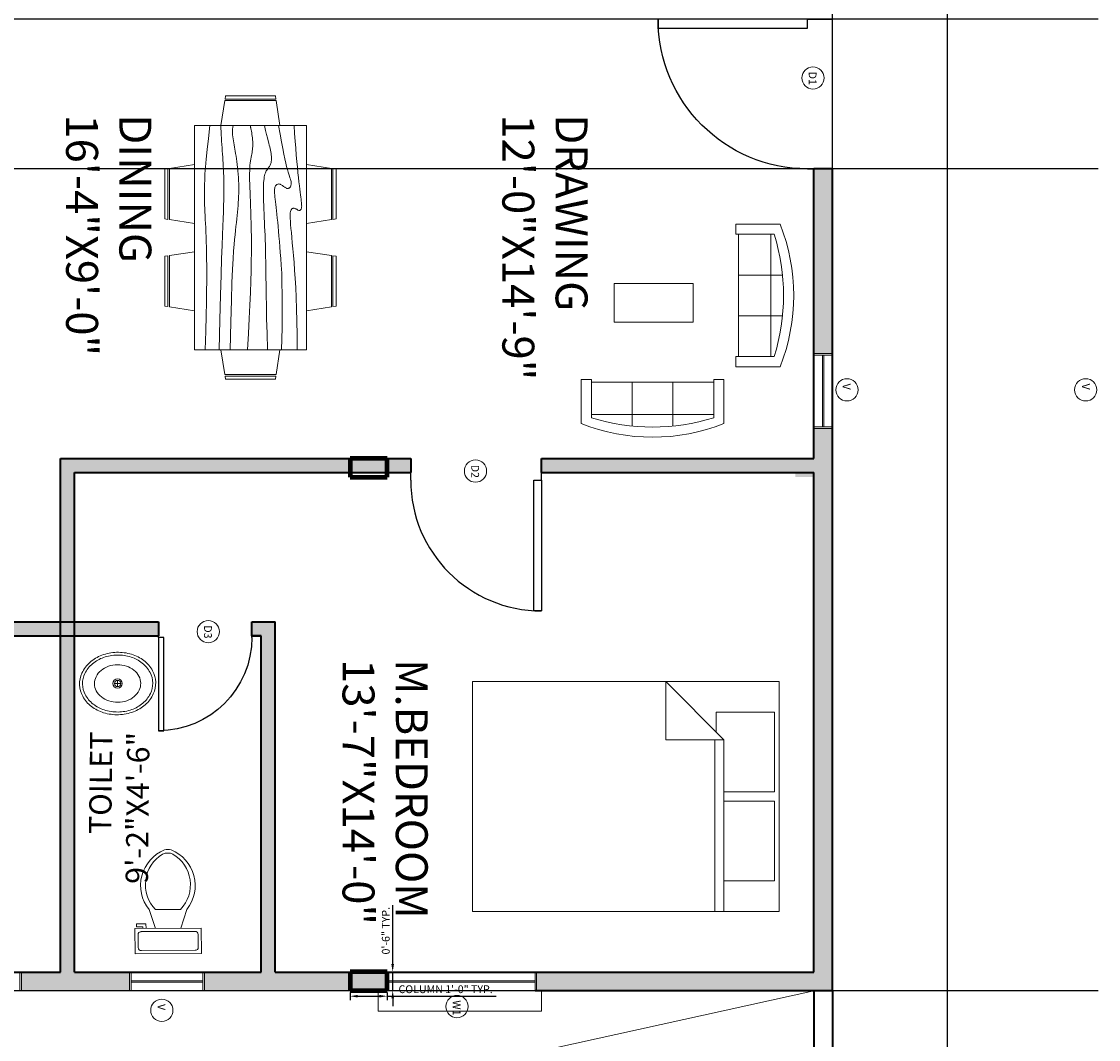
# Model space of a CAD drawing. Units: inches. Extents: x 7028582 to 7030319, y 63109697 to 63111305.
# Tile 10 of 18: x 7029402 to 7029748, y 63110530 to 63110857. Entities that reach past the tile are written whole.
import ezdxf

# ---------------------------------------------------------------- set-up
doc = ezdxf.new("R2010")
doc.units = ezdxf.units.IN
for name, color, linetype, lineweight in [('A-AREA-IDEN', 7, 'Continuous', 18), ('A-DOOR-IDEN', 20, 'Continuous', 13), ('A-FLOR-FIXT', 9, 'Continuous', 18), ('A-FLOR-OPEN', 7, 'Continuous', 13), ('A-GLAZ-IDEN', 20, 'Continuous', 13), ('A-WALL-PATT', 8, 'Continuous', 13), ('C-ANNO-DIMS', 7, 'Continuous', 18), ('doors', 20, 'Continuous', 25), ('furniture', 9, 'Continuous', 18), ('PILLARS', 220, 'Continuous', 100), ('S-COLS-PATT', 220, 'Continuous', 100), ('walls', 6, 'Continuous', 35), ('WINDOW SHADOW', 9, 'Continuous', 13), ('windows', 5, 'Continuous', 18)]:
    doc.layers.add(name, color=color, linetype=linetype, lineweight=lineweight)
doc.styles.get("Standard").update_dxf_attribs({"font": 'arial.ttf'})
doc.dimstyles.new('ISO-25', dxfattribs={"dimtxt": 2.5, "dimasz": 2.5, "dimexe": 1.25, "dimexo": 0.625, "dimtad": 1, "dimlunit": 4, "dimtxsty": 'Standard', "dimcen": 2.5, "dimadec": 0, "dimazin": 0, "dimtfac": 1, "dimtmove": 0, "dimatfit": 3, "dimfxl": 1, "dimarcsym": 0})

# ---------------------------------------------------------------- blocks, each defined once
blk = doc.blocks.new('*U2')
for p, q in [((0, 0), (0, -5)), ((30, 0), (30, -5))]:
    blk.add_line(p, q)
blk.add_lwpolyline([(0, 0), (0, 30), (1.75, 30), (1.75, 0)], close=True)
blk.add_arc((0, 0), 30, 0, 90)
blk = doc.blocks.new('Dining Set - 36 x 72 in.')
for p, q in [((-22.2343, 26.00059), (-23.4847, 17.99762)), ((-22.2304, 26), (-5.7608, 26)), ((-22, 27.5), (-22.1562, 26.50042)), ((-5.8416, 26.5), (-22.1534, 26.5)), ((-22, 27.5), (-6, 27.5)), ((-5.8437, 26.49966), (-6, 27.5)), ((-4.5152, 17.99762), (-5.7655, 25.99926)), ((5.7657, 26.00059), (4.5153, 17.99762)), ((5.7696, 26), (22.2392, 26)), ((6, 27.5), (5.8438, 26.50042)), ((22.1584, 26.5), (5.8466, 26.5)), ((6, 27.5), (22, 27.5)), ((22.1563, 26.49966), (22, 27.5)), ((23.4848, 17.99762), (22.2345, 25.99926)), ((36, 18), (-36, 18)), ((-36, 18), (-36, -18)), ((36, -18), (36, 18)), ((-45.5, 8), (-44.5004, 8.15617)), ((-45.5, 8), (-45.5, -8)), ((-44.5, -8.15843), (-44.5, 8.15338)), ((-44.0006, 8.23428), (-35.9976, 9.48474)), ((-44, 8.23041), (-44, -8.23915)), ((44.0006, 8.23428), (35.9976, 9.48474)), ((44, 8.23041), (44, -8.23915)), ((44.5, -8.15843), (44.5, 8.15338)), ((45.5, 8), (44.5005, 8.15617)), ((45.5, 8), (45.5, -8)), ((-44.4997, -8.15631), (-45.5, -8)), ((-35.9976, -9.48476), (-43.9993, -8.2345)), ((35.9976, -9.48476), (43.9993, -8.2345)), ((44.4997, -8.15631), (45.5, -8)), ((-36, -18), (36, -18)), ((-22.2343, -26.0006), (-23.4847, -17.99762)), ((-4.5152, -17.99762), (-5.7655, -25.99928)), ((5.7657, -26.0006), (4.5153, -17.99762)), ((23.4848, -17.99762), (22.2345, -25.99928)), ((-22.2304, -26), (-5.7608, -26)), ((-22, -27.5), (-22.1562, -26.50044)), ((-5.8416, -26.5), (-22.1534, -26.5)), ((-22, -27.5), (-6, -27.5)), ((-5.8437, -26.49967), (-6, -27.5)), ((5.7696, -26), (22.2392, -26)), ((6, -27.5), (5.8438, -26.50044)), ((22.1584, -26.5), (5.8466, -26.5)), ((6, -27.5), (22, -27.5)), ((22.1563, -26.49967), (22, -27.5))]:
    blk.add_line(p, q)
for points in [[(-36, 15), (-31.1772, 14.97754), (-26.8079, 14.91406), (-22.8538, 14.81543), (-19.276, 14.6875), (-16.0362, 14.53613), (-13.0957, 14.36718), (-10.4159, 14.18652), (-7.9583, 14), (-5.6904, 13.81315), (-3.6035, 13.63021), (-1.6954, 13.45508), (0.0365, 13.29166), (1.5945, 13.14388), (2.9811, 13.01562), (4.1988, 12.9108), (5.25, 12.83333), (6.1393, 12.78613), (6.8802, 12.76823), (7.4883, 12.77767), (7.9792, 12.8125), (8.3685, 12.87077), (8.6719, 12.95052), (8.9049, 13.0498), (9.0833, 13.16666), (9.2205, 13.29899), (9.3216, 13.44401), (9.3895, 13.59879), (9.4271, 13.76041), (9.4373, 13.92594), (9.4232, 14.09245), (9.3875, 14.257), (9.3333, 14.41666), (9.2638, 14.56917), (9.1836, 14.71484), (9.0975, 14.85465), (9.0104, 14.98958), (8.9272, 15.1206), (8.8529, 15.2487), (8.7922, 15.37483), (8.75, 15.5), (8.7305, 15.62467), (8.7344, 15.74739), (8.7617, 15.86621), (8.8125, 15.97916), (8.8867, 16.08431), (8.9844, 16.17968), (9.1055, 16.26334), (9.25, 16.33333), (9.4189, 16.38802), (9.6172, 16.42708), (9.8506, 16.45052), (10.125, 16.45833), (10.4463, 16.45052), (10.8203, 16.42708), (11.2529, 16.38802), (11.75, 16.33333), (12.3184, 16.26318), (12.9694, 16.17838), (13.7151, 16.07991), (14.5677, 15.96875), (15.5395, 15.84586), (16.6426, 15.71224), (17.8893, 15.56884), (19.2917, 15.41666), (20.859, 15.25667), (22.5879, 15.08984), (24.4721, 14.91715), (26.5052, 14.73958), (28.6809, 14.5581), (30.9929, 14.3737), (33.4347, 14.18733), (36, 14)], [(-36, 10), (-28.9766, 10.14274), (-23.1725, 10.20442), (-18.4241, 10.19775), (-14.5677, 10.13541), (-11.4399, 10.03011), (-8.877, 9.89453), (-6.7154, 9.74137), (-4.7917, 9.58333), (-2.9698, 9.43082), (-1.2246, 9.28515), (0.4415, 9.14534), (2.026, 9.01041), (3.5266, 8.87939), (4.9408, 8.7513), (6.266, 8.62516), (7.5, 8.5), (8.6411, 8.37549), (9.6914, 8.2539), (10.6538, 8.13818), (11.5312, 8.03125), (12.3267, 7.93603), (13.043, 7.85547), (13.6831, 7.79248), (14.25, 7.75), (14.7471, 7.7303), (15.1797, 7.73307), (15.5537, 7.75732), (15.875, 7.80208), (16.1494, 7.86637), (16.3828, 7.94922), (16.5811, 8.04964), (16.75, 8.16666), (16.8944, 8.29915), (17.0143, 8.44531), (17.1089, 8.60319), (17.1771, 8.77083), (17.218, 8.94629), (17.2305, 9.1276), (17.2137, 9.31282), (17.1667, 9.5), (17.0895, 9.6875), (16.987, 9.875), (16.8649, 10.0625), (16.7292, 10.25), (16.5856, 10.4375), (16.4401, 10.625), (16.2985, 10.8125), (16.1667, 11), (16.05, 11.18733), (15.9518, 11.3737), (15.8752, 11.5581), (15.8229, 11.73958), (15.798, 11.91715), (15.8034, 12.08984), (15.842, 12.25667), (15.9167, 12.41666), (16.0295, 12.56836), (16.1784, 12.70833), (16.3605, 12.83268), (16.5729, 12.9375), (16.8127, 13.01888), (17.0768, 13.07291), (17.3625, 13.0957), (17.6667, 13.08333), (17.9894, 13.03312), (18.3418, 12.94726), (18.7382, 12.82918), (19.1927, 12.68229), (19.7195, 12.51001), (20.3327, 12.31575), (21.0465, 12.10294), (21.875, 11.875), (22.8357, 11.63354), (23.959, 11.37304), (25.2786, 11.08618), (26.8282, 10.76562), (28.6414, 10.40405), (30.752, 9.99414), (33.1936, 9.52856), (36, 9)], [(-36, 5.5), (-30.7157, 5.3348), (-26.069, 5.20963), (-21.9946, 5.11767), (-18.4271, 5.05208), (-15.3009, 5.00602), (-12.5508, 4.97265), (-10.1112, 4.94515), (-7.9167, 4.91666), (-5.909, 4.88167), (-4.0586, 4.83984), (-2.3429, 4.79215), (-0.7396, 4.73958), (0.7739, 4.6831), (2.22, 4.6237), (3.6213, 4.56233), (5, 4.5), (6.373, 4.43782), (7.7344, 4.3776), (9.0723, 4.32129), (10.375, 4.27083), (11.6309, 4.22819), (12.8281, 4.19531), (13.9551, 4.17415), (15, 4.16666), (15.954, 4.17448), (16.819, 4.19791), (17.6001, 4.23698), (18.3021, 4.29166), (18.9299, 4.36198), (19.4883, 4.44791), (19.9823, 4.54948), (20.4167, 4.66666), (20.7969, 4.79899), (21.1302, 4.94401), (21.4245, 5.09879), (21.6875, 5.26041), (21.9271, 5.42594), (22.1511, 5.59245), (22.3672, 5.757), (22.5834, 5.91666), (22.8065, 6.06868), (23.0404, 6.21093), (23.2879, 6.34147), (23.5521, 6.45833), (23.8358, 6.55957), (24.142, 6.64323), (24.4735, 6.70735), (24.8334, 6.75), (25.2235, 6.76969), (25.642, 6.76692), (26.0858, 6.74267), (26.5521, 6.69791), (27.0379, 6.63362), (27.5404, 6.55078), (28.0565, 6.45036), (28.5834, 6.33333), (29.1242, 6.19987), (29.7071, 6.04687), (30.3661, 5.87044), (31.1354, 5.66666), (32.0493, 5.43164), (33.142, 5.16146), (34.4475, 4.85221), (36, 4.5)], [(-36, -1), (-30.7915, -0.6591), (-26.0195, -0.38216), (-21.6519, -0.16284), (-17.6563, 0.00521), (-14.0005, 0.12833), (-10.6523, 0.21289), (-7.5796, 0.26522), (-4.75, 0.29166), (-2.134, 0.29793), (0.2878, 0.28711), (2.5317, 0.26163), (4.6146, 0.22396), (6.5529, 0.17651), (8.3633, 0.12174), (10.0623, 0.06209), (11.6667, 0), (13.1899, -0.06201), (14.6341, -0.1211), (15.9982, -0.17432), (17.2813, -0.21875), (18.4823, -0.25147), (19.6003, -0.26953), (20.6343, -0.27002), (21.5834, -0.25), (22.4481, -0.20768), (23.2357, -0.14584), (23.9549, -0.06836), (24.6146, 0.02083), (25.2235, 0.11784), (25.7904, 0.21875), (26.3241, 0.31966), (26.8334, 0.41666), (27.3265, 0.50618), (27.8099, 0.58593), (28.2894, 0.65397), (28.7709, 0.70833), (29.2601, 0.74707), (29.763, 0.76823), (30.2855, 0.76985), (30.8334, 0.75), (31.4088, 0.70784), (31.9994, 0.64713), (32.589, 0.57275), (33.1615, 0.48958), (33.7008, 0.4025), (34.1908, 0.3164), (34.6153, 0.23616), (34.9584, 0.16666), (35.2099, 0.11165), (35.3848, 0.07031), (35.504, 0.04069), (35.5886, 0.02083), (35.6594, 0.00879), (35.7377, 0.0026), (35.8442, 0.00032), (36, 0)], [(-36, -6.5), (-27.1843, -6.31267), (-20.084, -6.1263), (-14.469, -5.9419), (-10.1094, -5.76042), (-6.7752, -5.58285), (-4.2363, -5.41016), (-2.2629, -5.24333), (-0.625, -5.08334), (0.8708, -4.93099), (2.2715, -4.78646), (3.5872, -4.64974), (4.8281, -4.52084), (6.0046, -4.39974), (7.127, -4.28646), (8.2053, -4.18099), (9.25, -4.08334), (10.2705, -3.99382), (11.2734, -3.91407), (12.2647, -3.84603), (13.25, -3.79167), (14.2354, -3.75293), (15.2266, -3.73177), (16.2295, -3.73015), (17.25, -3.75), (18.2912, -3.79248), (19.3451, -3.85547), (20.4009, -3.93604), (21.4479, -4.03125), (22.4754, -4.13819), (23.4727, -4.25391), (24.4289, -4.37549), (25.3334, -4.5), (26.1785, -4.62492), (26.9694, -4.74935), (27.7145, -4.87281), (28.4219, -4.99479), (29.1, -5.11483), (29.7572, -5.23242), (30.4016, -5.34709), (31.0417, -5.45834), (31.6837, -5.56437), (32.3262, -5.65821), (32.9658, -5.73153), (33.599, -5.77604), (34.2224, -5.78345), (34.8327, -5.74545), (35.4264, -5.65373), (36, -5.5)], [(-36, -10), (-26.4022, -9.81299), (-18.4675, -9.62891), (-11.9839, -9.45069), (-6.7396, -9.28125), (-2.5226, -9.12354), (0.8789, -8.98047), (3.6769, -8.85498), (6.0833, -8.75), (8.2767, -8.66765), (10.3021, -8.60677), (12.1712, -8.56543), (13.8958, -8.54167), (15.4876, -8.53353), (16.9583, -8.53907), (18.3197, -8.55632), (19.5834, -8.58334), (20.7616, -8.61841), (21.8685, -8.66081), (22.9188, -8.71004), (23.9271, -8.76563), (24.9081, -8.82707), (25.8763, -8.89388), (26.8465, -8.96558), (27.8334, -9.04167), (28.8474, -9.12118), (29.8828, -9.20117), (30.93, -9.27824), (31.9792, -9.34896), (33.0205, -9.40991), (34.0443, -9.45768), (35.0407, -9.48885), (36, -9.5)], [(-36, -14.5), (-30.0881, -14.33513), (-25.0332, -14.21224), (-20.7312, -14.12647), (-17.0781, -14.07292), (-13.97, -14.04671), (-11.3027, -14.04297), (-8.9724, -14.05681), (-6.875, -14.08334), (-4.9224, -14.11833), (-3.0905, -14.16016), (-1.3709, -14.20785), (0.2448, -14.26042), (1.7647, -14.3169), (3.1973, -14.3763), (4.5507, -14.43767), (5.8333, -14.5), (7.0554, -14.5621), (8.235, -14.62175), (9.3922, -14.67652), (10.5469, -14.72396), (11.7192, -14.76164), (12.929, -14.78711), (14.1965, -14.79794), (15.5417, -14.79167), (16.9933, -14.76424), (18.6152, -14.70508), (20.4804, -14.60197), (22.6615, -14.44271), (25.2312, -14.21509), (28.2624, -13.9069), (31.8277, -13.50594), (36, -13)]]:
    blk.add_lwpolyline(points)
blk = doc.blocks.new('Sofa - Roundback 7 ft.')
for p, q in [((-36.000027, -34), (-36.000027, -11.4696)), ((-12.00002, -32.4421), (-12.00003, -6.5971)), ((11.99997, -32.4421), (11.99998, -6.5971)), ((35.99998, -34), (35.99998, -11.4696)), ((-35.999844, -13.3819), (35.9998, -13.3819)), ((-36.000027, -32.4421), (35.99998, -32.4421))]:
    blk.add_line(p, q)
for points in [[(-36.000027, -34), (-42.000027, -34), (-42.000027, -8)], [(41.99998, -8), (41.99998, -34), (35.99998, -34)]]:
    blk.add_lwpolyline(points)
for centre, radius, start, end in [((0, -114.25), 114.25, 68.43141, 111.5686), ((-0.00001, -127.1968), 121.1968, 72.72033, 107.2797)]:
    blk.add_arc(centre, radius, start, end)
blk = doc.blocks.new('Toilet - top')
for p, q in [((9.5, -6), (9.5, -2)), ((-10, -8.5), (-8, -8.5)), ((-10, -9.5), (-10, -8.5)), ((-7, -9.5), (-10, -9.5)), ((-8, -8.5), (-8, -8)), ((-7, -8), (-7, -9.5)), ((-4, -8), (-6, -14)), ((4, -8), (6, -14)), ((4, -14), (-4, -14))]:
    blk.add_line(p, q)
blk.add_lwpolyline([(10.5, -8), (10.5, 0), (-10.5, 0), (-10.5, -8)], close=True)
for points in [[(-9.5, -2), (-9.5, -6)], [(8.5, -1), (-8.5, -1)], [(-8.5, -7), (8.5, -7)]]:
    blk.add_lwpolyline(points)
for centre, radius, start, end in [((-8.62, -1.88), 0.884, 81.8699, 188.1301), ((8.62, -1.88), 0.884, 351.8699, 98.1301), ((-8.62, -6.12), 0.884, 171.8699, 278.1301), ((8.62, -6.12), 0.884, 261.8699, 8.1301), ((3.52, -21.58), 12.17, 141.4691, 247.9714), ((4.2, -21.82), 11.33, 136.3677, 238.9468), ((-3.52, -21.58), 12.17, 292.0284, 38.5307), ((-4.2, -21.82), 11.33, 301.053, 43.6321), ((0, -27.88), 4, 245.7318, 294.2682), ((0, -29), 4, 254.8605, 285.1395)]:
    blk.add_arc(centre, radius, start, end)
blk = doc.blocks.new('Sink - Oval top')
for p, q in [((-1, 0), (1, 0)), ((0, 1), (0, -1))]:
    blk.add_line(p, q)
for points in [[(-12.23, 0.39, 0.117634), (-11.46, -3.36, 0.104469), (-8.88, -6.8, 0.090016), (-5.08, -9.07, 0.08192), (-0.32, -10.02, 0.08192), (4.49, -9.38, 0.090016), (8.42, -7.36, 0.104469), (11.22, -4.09, 0.117634), (12.23, -0.39, 0.117634), (11.46, 3.36, 0.104469), (8.88, 6.8, 0.090016), (5.08, 9.07, 0.08192), (0.32, 10.02, 0.08192), (-4.49, 9.38, 0.090016), (-8.42, 7.36, 0.104469), (-11.22, 4.09, 0.117634)], [(-11.29, 0.16, 0.118622), (-10.52, -3.25, 0.104678), (-8.07, -6.36, 0.089562), (-4.54, -8.37, 0.081185), (-0.13, -9.15, 0.081185), (4.3, -8.49, 0.089562), (7.89, -6.58, 0.104678), (10.42, -3.55, 0.118622), (11.29, -0.16, 0.118622), (10.52, 3.25, 0.104678), (8.07, 6.36, 0.089562), (4.54, 8.37, 0.081185), (0.13, 9.15, 0.081185), (-4.3, 8.49, 0.089562), (-7.89, 6.58, 0.104678), (-10.42, 3.55, 0.118622)], [(-7.42, 0.08, 0.118283), (-6.91, -2.17, 0.104607), (-5.29, -4.21, 0.089718), (-2.97, -5.53, 0.081436), (-0.07, -6.04, 0.081436), (2.84, -5.59, 0.089718), (5.2, -4.33, 0.104607), (6.86, -2.32, 0.118283), (7.42, -0.08, 0.118283), (6.91, 2.17, 0.104607), (5.29, 4.21, 0.089718), (2.97, 5.53, 0.081436), (0.07, 6.04, 0.081436), (-2.84, 5.59, 0.089718), (-5.2, 4.33, 0.104607), (-6.86, 2.32, 0.118283)]]:
    blk.add_lwpolyline(points, format="xyb", close=True)
for radius in [1.5, 1]:
    blk.add_circle((0, 0), radius)
blk = doc.blocks.new('Bed - Queen')
for p, q in [((0, -80.00003), (0, 0)), ((0, 0), (59.99999, 0)), ((59.99999, 0), (59.99999, -80.00003)), ((7.99999, -1.2), (28.79998, -1.2)), ((7.99999, -14.4), (7.99999, -1.2)), ((28.79998, -1.2), (28.79998, -14.4)), ((31.19999, -1.2), (51.99999, -1.2)), ((31.19999, -14.4), (31.19999, -1.2)), ((51.99999, -1.2), (51.99999, -16.4)), ((0, -14.4), (44.8, -14.4)), ((44.8, -16.8), (0, -16.8)), ((59.99999, -29.6), (44.8, -14.4)), ((44.8, -14.4), (44.8, -29.6)), ((51.99999, -16.4), (46.79936, -16.4)), ((44.8, -29.6), (59.99999, -29.6)), ((59.99999, -80.00003), (0, -80.00003))]:
    blk.add_line(p, q)
blk = doc.blocks.new('WIN-SASH-24')
for p, q in [((24.05, 6), (0, 6)), ((0.5, 6), (0.5, 0)), ((23.55, 0), (23.55, 6)), ((0, 0), (24.05, 0)), ((23.55, 3.2), (0.5, 3.2)), ((23.55, 2.8), (0.5, 2.8))]:
    blk.add_line(p, q)
blk = doc.blocks.new('WIN-SASH-24-FRAME')
for p, q in [((24.05, 6), (0, 6)), ((0.5, 6), (0.5, 0)), ((23.55, 0), (23.55, 6)), ((0, 0), (24.05, 0))]:
    blk.add_line(p, q)
blk = doc.blocks.new('WIN-SASH-48')
for p, q in [((48.05, 6), (0, 6)), ((0.5, 6), (0.5, 0)), ((47.55, 0), (47.55, 6)), ((47.55, 3.2), (0.5, 3.2)), ((47.55, 2.8), (0.5, 2.8)), ((0, 0), (48.05, 0))]:
    blk.add_line(p, q)
blk = doc.blocks.new('WINDOW-SHADE-COURT-52')
for p, q in [((0, 0), (0, 6.54)), ((52.45, 6.54), (52.45, 0)), ((52.45, 0), (0, 0))]:
    blk.add_line(p, q)
blk = doc.blocks.new('COLUMN-RECT-PROFILE')
for p, q in [((11.91, 6), (0, 6)), ((0, 6), (0, 0)), ((11.91, 0), (11.91, 6)), ((0, 0), (11.91, 0))]:
    blk.add_line(p, q)
blk = doc.blocks.new('TABLE-COFFEE-RECT')
blk.add_lwpolyline([(25.34, 12.34), (0, 12.34), (0, 0), (25.34, 0)], close=True)
blk = doc.blocks.new('TAG-V-MT-R')
blk.add_circle((3.58, 3.58), 3.58)
at = {"insert": (4.93, 5.6), "char_height": 2.5, "attachment_point": 1, "rotation": 270}
blk.add_mtext_dynamic_manual_height_columns('V', width=2.5021, gutter_width=12.5, heights=[0], dxfattribs=at)
blk = doc.blocks.new('TAG-D2-MT-L')
blk.add_circle((3.58, 3.58), 3.58)
at = {"insert": (2.23, 5.6), "char_height": 2.5, "attachment_point": 7, "rotation": 270}
blk.add_mtext_dynamic_manual_height_columns('D2', width=2.5021, gutter_width=12.5, heights=[0], dxfattribs=at)
blk = doc.blocks.new('TAG-D3-MT-L')
blk.add_circle((3.58, 3.58), 3.58)
at = {"insert": (2.23, 5.6), "char_height": 2.5, "attachment_point": 7, "rotation": 270}
blk.add_mtext_dynamic_manual_height_columns('D3', width=2.5021, gutter_width=12.5, heights=[0], dxfattribs=at)
blk = doc.blocks.new('TAG-V-MT-L')
blk.add_circle((3.58, 3.58), 3.58)
at = {"insert": (2.23, 5.6), "char_height": 2.5, "attachment_point": 7, "rotation": 270}
blk.add_mtext_dynamic_manual_height_columns('V', width=2.5021, gutter_width=12.5, heights=[0], dxfattribs=at)
blk = doc.blocks.new('TAG-W1-MT-L')
blk.add_circle((3.58, 3.58), 3.58)
at = {"insert": (2.23, 5.6), "char_height": 2.5, "attachment_point": 7, "rotation": 270}
blk.add_mtext_dynamic_manual_height_columns('W1', width=2.5021, gutter_width=12.5, heights=[0], dxfattribs=at)
blk = doc.blocks.new('*D47')
at = {"layer": 'C-ANNO-DIMS', "color": 0, "lineweight": -2, "transparency": 16777216}
for p, q in [((7029507.24, 63110544.98), (7029507.24, 63110542.57)), ((7029519.15, 63110544.98), (7029519.15, 63110542.57)), ((7029509.74, 63110543.82), (7029516.65, 63110543.82)), ((7029519.15, 63110543.82), (7029554.22, 63110543.82))]:
    blk.add_line(p, q, dxfattribs=at)
at = {"layer": 'C-ANNO-DIMS', "color": 0, "lineweight": 100, "transparency": 16777216}
for points in [[(7029509.74, 63110544.24), (7029509.74, 63110543.4), (7029507.24, 63110543.82)], [(7029516.65, 63110544.24), (7029516.65, 63110543.4), (7029519.15, 63110543.82)]]:
    blk.add_solid(points, dxfattribs=at)
at = {"layer": 'Defpoints', "color": 0, "lineweight": 100, "transparency": 16777216}
for p in [(7029507.24, 63110545.61), (7029519.15, 63110545.61), (7029519.15, 63110543.82)]:
    blk.add_point(p, dxfattribs=at)
at = {"layer": 'C-ANNO-DIMS', "color": 0, "transparency": 16777216, "insert": (7029537.94, 63110545.74), "char_height": 2.5, "attachment_point": 5}
blk.add_mtext('COLUMN 1\'-0" TYP.', dxfattribs=at)
blk = doc.blocks.new('*D48')
at = {"layer": 'C-ANNO-DIMS', "color": 0, "lineweight": -2, "transparency": 16777216}
for p, q in [((7029520.94, 63110554.11), (7029520.94, 63110573.1)), ((7029519.78, 63110551.61), (7029522.19, 63110551.61)), ((7029520.94, 63110545.61), (7029520.94, 63110551.61)), ((7029519.78, 63110545.61), (7029522.19, 63110545.61)), ((7029520.94, 63110543.11), (7029520.94, 63110540.61))]:
    blk.add_line(p, q, dxfattribs=at)
at = {"layer": 'C-ANNO-DIMS', "color": 0, "lineweight": 100, "transparency": 16777216}
for points in [[(7029520.52, 63110554.11), (7029521.36, 63110554.11), (7029520.94, 63110551.61)], [(7029520.52, 63110543.11), (7029521.36, 63110543.11), (7029520.94, 63110545.61)]]:
    blk.add_solid(points, dxfattribs=at)
at = {"layer": 'Defpoints', "color": 0, "lineweight": 100, "transparency": 16777216}
for p in [(7029519.15, 63110551.61), (7029520.94, 63110551.61), (7029519.15, 63110545.61)]:
    blk.add_point(p, dxfattribs=at)
at = {"layer": 'C-ANNO-DIMS', "color": 0, "transparency": 16777216, "insert": (7029519.04, 63110564.85), "char_height": 2.5, "attachment_point": 5, "rotation": 90}
blk.add_mtext('0\'-6" TYP.', dxfattribs=at)
blk = doc.blocks.new('*D104')
at = {"layer": 'C-ANNO-DIMS', "color": 0, "lineweight": -2, "transparency": 16777216}
for p, q in [((7029747.58, 63110857.56), (7028586.23, 63110857.56)), ((7028587.48, 63110812.06), (7028587.48, 63110855.06)), ((7029747.58, 63110809.56), (7028586.23, 63110809.56))]:
    blk.add_line(p, q, dxfattribs=at)
at = {"layer": 'C-ANNO-DIMS', "color": 0, "lineweight": 100, "transparency": 16777216}
for points in [[(7028587.06, 63110855.06), (7028587.89, 63110855.06), (7028587.48, 63110857.56)], [(7028587.06, 63110812.06), (7028587.89, 63110812.06), (7028587.48, 63110809.56)]]:
    blk.add_solid(points, dxfattribs=at)
at = {"layer": 'Defpoints', "color": 0, "lineweight": 100, "transparency": 16777216}
for p in [(7028587.48, 63110857.56), (7029748.21, 63110857.56), (7029748.21, 63110809.56)]:
    blk.add_point(p, dxfattribs=at)
at = {"layer": 'C-ANNO-DIMS', "color": 0, "transparency": 16777216, "insert": (7028585.57, 63110833.56), "char_height": 2.5, "attachment_point": 5, "rotation": 90}
blk.add_mtext('4\'-0"', dxfattribs=at)
blk = doc.blocks.new('*D108')
at = {"layer": 'C-ANNO-DIMS', "color": 0, "lineweight": -2, "transparency": 16777216}
for p, q in [((7029662.21, 63110129.18), (7029662.21, 63111300.44)), ((7029664.71, 63111299.19), (7029696.71, 63111299.19)), ((7029699.21, 63110129.18), (7029699.21, 63111300.44))]:
    blk.add_line(p, q, dxfattribs=at)
at = {"layer": 'C-ANNO-DIMS', "color": 0, "lineweight": 100, "transparency": 16777216}
for points in [[(7029664.71, 63111299.61), (7029664.71, 63111298.77), (7029662.21, 63111299.19)], [(7029696.71, 63111299.61), (7029696.71, 63111298.77), (7029699.21, 63111299.19)]]:
    blk.add_solid(points, dxfattribs=at)
at = {"layer": 'Defpoints', "color": 0, "lineweight": 100, "transparency": 16777216}
for p in [(7029699.21, 63111299.19), (7029662.21, 63110128.56), (7029699.21, 63110128.56)]:
    blk.add_point(p, dxfattribs=at)
at = {"layer": 'C-ANNO-DIMS', "color": 0, "transparency": 16777216, "insert": (7029680.71, 63111301.09), "char_height": 2.5, "attachment_point": 5}
blk.add_mtext('3\'-1"', dxfattribs=at)
blk = doc.blocks.new('*D112')
at = {"layer": 'C-ANNO-DIMS', "color": 0, "lineweight": -2, "transparency": 16777216}
for p, q in [((7029747.58, 63111033.06), (7028586.23, 63111033.06)), ((7028587.48, 63111030.56), (7028587.48, 63110548.06)), ((7029747.58, 63110545.56), (7028586.23, 63110545.56))]:
    blk.add_line(p, q, dxfattribs=at)
at = {"layer": 'C-ANNO-DIMS', "color": 0, "lineweight": 100, "transparency": 16777216}
for points in [[(7028587.06, 63111030.56), (7028587.89, 63111030.56), (7028587.48, 63111033.06)], [(7028587.06, 63110548.06), (7028587.89, 63110548.06), (7028587.48, 63110545.56)]]:
    blk.add_solid(points, dxfattribs=at)
at = {"layer": 'Defpoints', "color": 0, "lineweight": 100, "transparency": 16777216}
for p in [(7029748.21, 63111033.06), (7028587.48, 63110545.56), (7029748.21, 63110545.56)]:
    blk.add_point(p, dxfattribs=at)
at = {"layer": 'C-ANNO-DIMS', "color": 0, "transparency": 16777216, "insert": (7028585.56, 63110789.31), "char_height": 2.5, "attachment_point": 5, "rotation": 90}
blk.add_mtext('40\'-7 1/2"', dxfattribs=at)

msp = doc.modelspace()

# ---------------------------------------------------------------- hatches: boundary and pattern name
at = {"layer": 'A-WALL-PATT'}
h = msp.add_hatch(color=256, dxfattribs=at)
h.dxf.hatch_style = 1
h.paths.add_polyline_path([(7029656.205, 63110809.557), (7029662.205, 63110809.557), (7029662.205, 63110750.186), (7029656.205, 63110750.186)])
h = msp.add_hatch(color=256, dxfattribs=at)
h.dxf.hatch_style = 1
h.paths.add_polyline_path([(7029567.185, 63110551.557), (7029567.185, 63110545.557), (7029662.205, 63110545.557), (7029662.205, 63110726.137), (7029656.205, 63110726.137), (7029656.205, 63110716.557), (7029568.726, 63110716.557), (7029568.726, 63110712.057), (7029656.205, 63110712.057), (7029656.205, 63110551.557)])
h = msp.add_hatch(color=256, dxfattribs=at)
h.dxf.hatch_style = 1
h.paths.add_polyline_path([(7029568.726, 63110716.557), (7029656.205, 63110716.557), (7029656.205, 63110726.137), (7029662.205, 63110726.137), (7029662.205, 63110545.557), (7029572.732, 63110545.557), (7029572.732, 63110551.557), (7029656.205, 63110551.557), (7029656.205, 63110712.057), (7029568.726, 63110712.057)])
h = msp.add_hatch(color=256, dxfattribs=at)
h.dxf.hatch_style = 1
h.paths.add_polyline_path([(7029414.205, 63110716.557), (7029414.205, 63110664.057), (7029418.705, 63110664.057), (7029418.705, 63110712.057), (7029526.726, 63110712.057), (7029526.726, 63110716.557)])
h = msp.add_hatch(color=256, dxfattribs=at)
h.dxf.hatch_style = 1
h.paths.add_polyline_path([(7029414.205, 63110659.557), (7029414.205, 63110664.057), (7029360.705, 63110664.057), (7029360.705, 63110656.557), (7029365.205, 63110656.557), (7029365.205, 63110659.557)])
h = msp.add_hatch(color=256, dxfattribs=at)
h.dxf.hatch_style = 1
h.paths.add_polyline_path([(7029414.205, 63110664.057), (7029418.705, 63110664.057), (7029418.705, 63110659.557), (7029414.205, 63110659.557)])
h = msp.add_hatch(color=256, dxfattribs=at)
h.dxf.hatch_style = 1
h.paths.add_polyline_path([(7029418.705, 63110664.057), (7029445.705, 63110664.057), (7029445.705, 63110659.557), (7029418.705, 63110659.557)])
h = msp.add_hatch(color=256, dxfattribs=at)
h.dxf.hatch_style = 1
h.paths.add_polyline_path([(7029519.136, 63110545.557), (7029519.136, 63110551.557), (7029483.205, 63110551.557), (7029483.205, 63110664.057), (7029475.705, 63110664.057), (7029475.705, 63110659.557), (7029478.705, 63110659.557), (7029478.705, 63110551.557), (7029460.479, 63110551.557), (7029460.479, 63110545.557)])
h = msp.add_hatch(color=256, dxfattribs=at)
h.dxf.hatch_style = 1
h.paths.add_polyline_path([(7029414.205, 63110659.557), (7029414.205, 63110551.557), (7029401.714, 63110551.557), (7029401.714, 63110545.557), (7029436.431, 63110545.557), (7029436.431, 63110551.557), (7029418.705, 63110551.557), (7029418.705, 63110659.557)])
at = {"layer": 'S-COLS-PATT'}
h = msp.add_hatch(color=256, dxfattribs=at)
h.dxf.hatch_style = 1
h.paths.add_polyline_path([(7029662.205, 63110716.557), (7029650.291, 63110716.557), (7029650.291, 63110710.557), (7029662.205, 63110710.557)])
h = msp.add_hatch(color=256, dxfattribs=at)
h.dxf.hatch_style = 1
h.paths.add_polyline_path([(7029662.205, 63110551.607), (7029650.291, 63110551.607), (7029650.291, 63110545.607), (7029662.205, 63110545.607)])

# ---------------------------------------------------------------- linework, layer by layer
at = {"layer": 'A-DOOR-IDEN'}
msp.add_circle((7029655.936, 63110838.719), 3.577, dxfattribs=at)
at = {"layer": 'A-FLOR-OPEN'}
msp.add_line((7029240.705, 63110454.057), (7029656.205, 63110545.557), dxfattribs=at)
at = {"layer": 'walls'}
for p, q in [((7029656.205, 63110716.557), (7029656.205, 63110809.557)), ((7029662.205, 63110809.557), (7029656.205, 63110809.557)), ((7029662.205, 63110545.557), (7029662.205, 63110809.557)), ((7029414.205, 63110551.557), (7029414.205, 63110716.557)), ((7029414.205, 63110716.557), (7029526.726, 63110716.557)), ((7029526.726, 63110716.557), (7029526.726, 63110712.057)), ((7029568.726, 63110716.557), (7029656.205, 63110716.557)), ((7029568.726, 63110712.057), (7029568.726, 63110716.557)), ((7029418.705, 63110551.557), (7029418.705, 63110712.057)), ((7029418.705, 63110712.057), (7029526.726, 63110712.057)), ((7029568.726, 63110712.057), (7029656.205, 63110712.057)), ((7029656.205, 63110551.557), (7029656.205, 63110712.057)), ((7029360.705, 63110664.057), (7029445.705, 63110664.057)), ((7029445.705, 63110664.057), (7029445.705, 63110659.557)), ((7029475.705, 63110664.057), (7029483.205, 63110664.057)), ((7029475.705, 63110659.557), (7029475.705, 63110664.057)), ((7029483.205, 63110551.557), (7029483.205, 63110664.057)), ((7029365.205, 63110659.557), (7029445.705, 63110659.557)), ((7029475.705, 63110659.557), (7029478.705, 63110659.557)), ((7029478.705, 63110659.557), (7029475.705, 63110659.557)), ((7029478.705, 63110551.557), (7029478.705, 63110659.557)), ((7029365.205, 63110551.557), (7029414.205, 63110551.557)), ((7029418.705, 63110551.557), (7029478.705, 63110551.557)), ((7029483.205, 63110551.557), (7029656.205, 63110551.557)), ((7029662.205, 63110545.557), (7029566.685, 63110545.557)), ((7029656.205, 63110545.557), (7029656.205, 63110448.057)), ((7029662.205, 63110545.557), (7029662.205, 63110542.557)), ((7029662.205, 63110542.557), (7029662.205, 63110457.057))]:
    msp.add_line(p, q, dxfattribs=at)
at = {"layer": 'windows'}
for p, q in [((7029656.205, 63110750.186), (7029662.205, 63110750.186)), ((7029662.205, 63110726.137), (7029656.205, 63110726.137)), ((7029401.714, 63110551.557), (7029401.714, 63110545.557)), ((7029436.431, 63110545.557), (7029436.431, 63110551.557)), ((7029460.479, 63110551.557), (7029460.479, 63110545.557)), ((7029519.136, 63110545.557), (7029519.136, 63110551.557)), ((7029567.185, 63110551.557), (7029567.185, 63110545.557))]:
    msp.add_line(p, q, dxfattribs=at)

# ---------------------------------------------------------------- block references
at = {"layer": 'A-DOOR-IDEN'}
for name, p in [('TAG-D2-MT-L', (7029543.956, 63110708.893)), ('TAG-D3-MT-L', (7029458.118, 63110657.328))]:
    msp.add_blockref(name, p, dxfattribs=at)
at = {"layer": 'A-FLOR-FIXT', "xscale": -1}
msp.add_blockref('Sink - Oval top', (7029432.582, 63110644.243), dxfattribs=at)
at = {"layer": 'A-FLOR-FIXT', "xscale": -1.013555723357934, "yscale": 1.013555723357934, "zscale": 1.013555723357934, "rotation": 180.274620379553}
msp.add_blockref('Toilet - top', (7029448.831, 63110557.497), dxfattribs=at)
at = {"layer": 'A-GLAZ-IDEN'}
for name, p in [('TAG-V-MT-L', (7029663.285, 63110734.979)), ('TAG-V-MT-R', (7029739.972, 63110734.979)), ('TAG-V-MT-L', (7029443.2, 63110535.713)), ('TAG-W1-MT-L', (7029538.009, 63110536.914))]:
    msp.add_blockref(name, p, dxfattribs=at)
at = {"layer": 'doors'}
for p, xscale, yscale, zscale, rotation in [((7029654.205, 63110857.557), -1.599999999999999, 1.599999999999999, 1.599999999999999, 90), ((7029568.726, 63110709.557), 1.399999999999999, 1.399999999999999, 1.399999999999999, 180)]:
    msp.add_blockref('*U2', p, dxfattribs=dict(at, xscale=xscale, yscale=yscale, zscale=zscale, rotation=rotation))
at = {"layer": 'doors', "xscale": -1, "rotation": 180}
msp.add_blockref('*U2', (7029445.705, 63110659.057), dxfattribs=at)
at = {"layer": 'furniture', "xscale": -1, "rotation": 270}
msp.add_blockref('Dining Set - 36 x 72 in.', (7029475.247, 63110787.448), dxfattribs=at)
at = {"layer": 'furniture'}
for name, p, xscale, yscale, zscale, rotation in [('Sofa - Roundback 7 ft.', (7029649.752, 63110768.875), -0.5455524879488546, 0.5455524879488546, 0.5455524879488546, 270), ('Sofa - Roundback 7 ft.', (7029604.428, 63110723.346), -0.5455524879488546, 0.5455524879488546, 0.5455524879488546, 180), ('Bed - Queen', (7029645.108, 63110571.002), -1.232093012797833, 1.232093012797833, 1.232093012797833, 270)]:
    msp.add_blockref(name, p, dxfattribs=dict(at, xscale=xscale, yscale=yscale, zscale=zscale, rotation=rotation))
at = {"layer": 'furniture', "extrusion": (0, 0, -1), "zscale": -1}
msp.add_blockref('TABLE-COFFEE-RECT', (-7029617.436, 63110760.346), dxfattribs=at)
at = {"layer": 'PILLARS'}
for p in [(7029507.238, 63110710.557), (7029507.238, 63110545.607)]:
    msp.add_blockref('COLUMN-RECT-PROFILE', p, dxfattribs=at)
at = {"layer": 'WINDOW SHADOW'}
msp.add_blockref('WINDOW-SHADE-COURT-52', (7029516.285, 63110539.016), dxfattribs=at)
at = {"layer": 'windows', "rotation": 269.9999999926617}
msp.add_blockref('WIN-SASH-24', (7029656.205, 63110750.186), dxfattribs=at)
at = {"layer": 'windows'}
for name, p in [('WIN-SASH-24-FRAME', (7029377.666, 63110545.557)), ('WIN-SASH-24', (7029436.431, 63110545.557)), ('WIN-SASH-48', (7029519.136, 63110545.557))]:
    msp.add_blockref(name, p, dxfattribs=at)

# ---------------------------------------------------------------- texts
at = {"layer": 'A-AREA-IDEN'}
for s, width, gutter_width, insert, char_height, attachment_point, rotation in [('DINING\\P16\'-4"X9\'-0"', 82.04322, 51.315, (7029416.035, 63110827.03), 10.26307, 7, 270), ('DRAWING\\P12\'-0"X14\'-9"', 82.04322, 51.315, (7029556.17, 63110827.03), 10.26307, 7, 270), ('M.BEDROOM\\P13\'-7"X14\'-0"', 82.04322, 51.315, (7029504.833, 63110652.083), 10.26307, 7, 270), ('TOILET\\P9\'-2"X4\'-6"', 42.97461, 35.821, (7029423.746, 63110628.835), 7.16426, 3, 89.3536)]:
    msp.add_mtext_dynamic_manual_height_columns(s, width=width, gutter_width=gutter_width, heights=[0], dxfattribs=dict(at, insert=insert, char_height=char_height, attachment_point=attachment_point, rotation=rotation))
at = {"layer": 'A-DOOR-IDEN', "insert": (7029654.584, 63110840.744), "char_height": 2.5, "attachment_point": 7, "rotation": 270}
msp.add_mtext_dynamic_manual_height_columns('D1', width=2.50214, gutter_width=12.5, heights=[0], dxfattribs=at)

# ---------------------------------------------------------------- dimensions: what is measured, and where the dimension line sits
at = {"layer": 'C-ANNO-DIMS'}
dim = msp.add_linear_dim(base=(7029699.205, 63111299.19), p1=(7029662.205, 63110128.557), p2=(7029699.205, 63110128.557), dimstyle='ISO-25', override={"dimdec": 1, "dimlfac": 1, "dimrnd": 0, "dimzin": 1, "dimdsep": 46, "dimlunit": 4, "dimfrac": 2}, dxfattribs=at)
dim.commit()
dim.dimension.update_dxf_attribs({"geometry": '*D108', "text_midpoint": (7029680.705, 63111301.092)})
for base, p1, p2, picture, middle in [((7028587.475, 63110545.557), (7029748.205, 63111033.057), (7029748.205, 63110545.557), '*D112', (7028585.558, 63110789.307)), ((7028587.475, 63110857.557), (7029748.205, 63110809.557), (7029748.205, 63110857.557), '*D104', (7028585.574, 63110833.557))]:
    dim = msp.add_linear_dim(base=base, p1=p1, p2=p2, angle=90, dimstyle='ISO-25', override={"dimdec": 1, "dimlfac": 1, "dimrnd": 0, "dimzin": 1, "dimdsep": 46, "dimlunit": 4, "dimfrac": 2}, dxfattribs=at)
    dim.commit()
    dim.dimension.update_dxf_attribs({"geometry": picture, "text_midpoint": middle})
dim = msp.add_linear_dim(base=(7029520.94, 63110551.607), p1=(7029519.153, 63110545.607), p2=(7029519.153, 63110551.607), angle=90, text='<> TYP.', dimstyle='ISO-25', override={"dimdec": 1, "dimlfac": 1, "dimrnd": 0, "dimzin": 1, "dimdsep": 46, "dimlunit": 4, "dimfrac": 2}, dxfattribs=at)
dim.commit()
dim.dimension.update_dxf_attribs({"geometry": '*D48', "text_midpoint": (7029519.039, 63110564.852)})
dim = msp.add_linear_dim(base=(7029519.153, 63110543.82), p1=(7029507.238, 63110545.607), p2=(7029519.153, 63110545.607), text='COLUMN <> TYP.', dimstyle='ISO-25', override={"dimdec": 1, "dimlfac": 1, "dimrnd": 0, "dimzin": 1, "dimdsep": 46, "dimlunit": 4, "dimfrac": 2}, dxfattribs=at)
dim.commit()
dim.dimension.update_dxf_attribs({"geometry": '*D47', "text_midpoint": (7029537.935, 63110545.738)})

doc.saveas('drawing.dxf')
